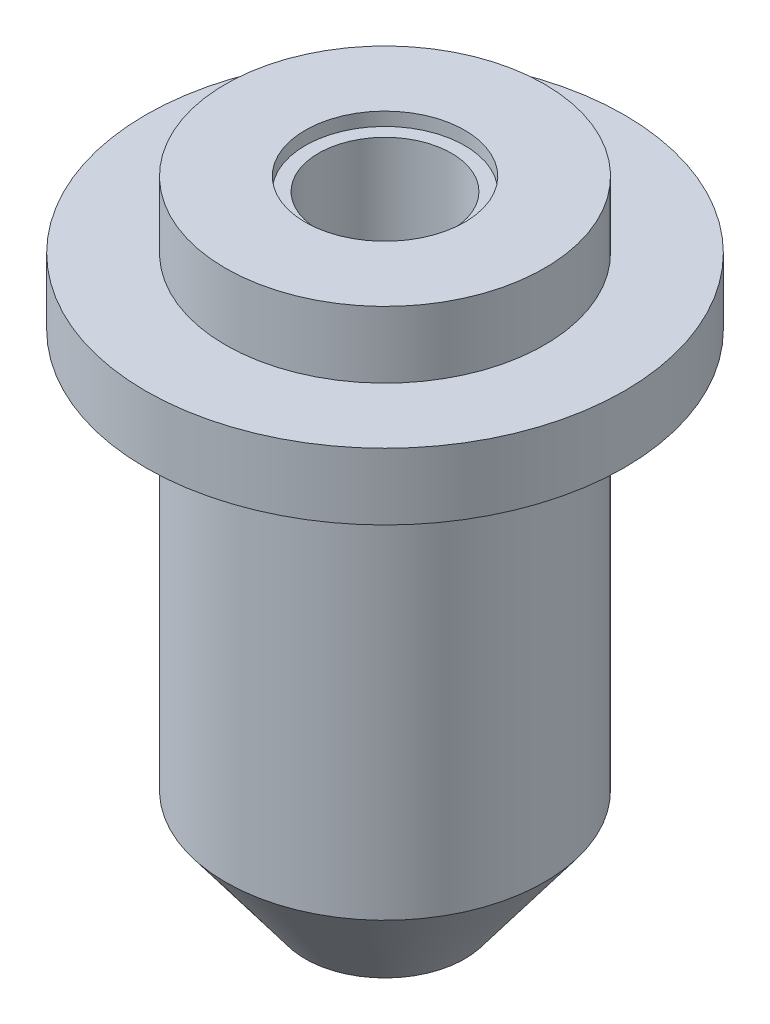
ISO-10303-21;
HEADER;
FILE_DESCRIPTION(('STEP AP214'),'2;1');
FILE_NAME('part.step','',(''),(''),'','','');
FILE_SCHEMA(('AUTOMOTIVE_DESIGN { 1 0 10303 214 1 1 1 1 }'));
ENDSEC;
DATA;
#1=APPLICATION_CONTEXT('core data for automotive mechanical design processes');
#2=APPLICATION_PROTOCOL_DEFINITION('international standard','automotive_design',2000,#1);
#3=PRODUCT_CONTEXT('',#1,'mechanical');
#4=PRODUCT('Part','Part','',(#3));
#5=PRODUCT_RELATED_PRODUCT_CATEGORY('part','',(#4));
#6=PRODUCT_DEFINITION_FORMATION('','',#4);
#7=PRODUCT_DEFINITION_CONTEXT('part definition',#1,'design');
#8=PRODUCT_DEFINITION('design','',#6,#7);
#9=PRODUCT_DEFINITION_SHAPE('','',#8);
#10=(LENGTH_UNIT() NAMED_UNIT(*) SI_UNIT(.MILLI.,.METRE.));
#11=(NAMED_UNIT(*) PLANE_ANGLE_UNIT() SI_UNIT($,.RADIAN.));
#12=(NAMED_UNIT(*) SI_UNIT($,.STERADIAN.) SOLID_ANGLE_UNIT());
#13=UNCERTAINTY_MEASURE_WITH_UNIT(LENGTH_MEASURE(1.E-05),#10,'distance_accuracy_value','');
#14=(GEOMETRIC_REPRESENTATION_CONTEXT(3) GLOBAL_UNCERTAINTY_ASSIGNED_CONTEXT((#13)) GLOBAL_UNIT_ASSIGNED_CONTEXT((#10,
#11,#12)) REPRESENTATION_CONTEXT('',''));
#15=CARTESIAN_POINT('',(0.,0.,0.));
#16=DIRECTION('',(0.,0.,1.));
#17=DIRECTION('',(1.,0.,0.));
#18=AXIS2_PLACEMENT_3D('',#15,#16,#17);
#19=CARTESIAN_POINT('',(0.,0.,0.));
#20=DIRECTION('',(0.,1.,0.));
#21=DIRECTION('',(0.,0.,1.));
#22=AXIS2_PLACEMENT_3D('',#19,#20,#21);
#23=PLANE('',#22);
#24=CARTESIAN_POINT('',(0.,0.,0.));
#25=DIRECTION('',(0.,1.,0.));
#26=DIRECTION('',(0.,0.,1.));
#27=AXIS2_PLACEMENT_3D('',#24,#25,#26);
#28=CIRCLE('',#27,5.);
#29=CARTESIAN_POINT('',(0.,0.,5.));
#30=VERTEX_POINT('',#29);
#31=EDGE_CURVE('E73',#30,#30,#28,.T.);
#32=ORIENTED_EDGE('',*,*,#31,.T.);
#33=EDGE_LOOP('',(#32));
#34=FACE_BOUND('',#33,.T.);
#35=CARTESIAN_POINT('',(0.,0.,0.));
#36=DIRECTION('',(0.,-1.,0.));
#37=DIRECTION('',(0.,0.,-1.));
#38=AXIS2_PLACEMENT_3D('',#35,#36,#37);
#39=CIRCLE('',#38,6.);
#40=CARTESIAN_POINT('',(0.,0.,-6.));
#41=VERTEX_POINT('',#40);
#42=EDGE_CURVE('E10',#41,#41,#39,.T.);
#43=ORIENTED_EDGE('',*,*,#42,.T.);
#44=EDGE_LOOP('',(#43));
#45=FACE_BOUND('',#44,.T.);
#46=ADVANCED_FACE('F43',(#34,#45),#23,.F.);
#47=CARTESIAN_POINT('',(0.,8.,0.));
#48=DIRECTION('',(0.,1.,0.));
#49=DIRECTION('',(0.,0.,1.));
#50=AXIS2_PLACEMENT_3D('',#47,#48,#49);
#51=CONICAL_SURFACE('',#50,12.,0.643501108793284);
#52=ORIENTED_EDGE('',*,*,#42,.F.);
#53=EDGE_LOOP('',(#52));
#54=FACE_BOUND('',#53,.T.);
#55=CARTESIAN_POINT('',(0.,8.,0.));
#56=DIRECTION('',(0.,-1.,0.));
#57=DIRECTION('',(0.,0.,-1.));
#58=AXIS2_PLACEMENT_3D('',#55,#56,#57);
#59=CIRCLE('',#58,12.);
#60=CARTESIAN_POINT('',(0.,8.,-12.));
#61=VERTEX_POINT('',#60);
#62=EDGE_CURVE('E47',#61,#61,#59,.T.);
#63=ORIENTED_EDGE('',*,*,#62,.T.);
#64=EDGE_LOOP('',(#63));
#65=FACE_BOUND('',#64,.T.);
#66=ADVANCED_FACE('F125',(#54,#65),#51,.T.);
#67=CARTESIAN_POINT('',(0.,0.,0.));
#68=DIRECTION('',(0.,-1.,0.));
#69=DIRECTION('',(0.,0.,-1.));
#70=AXIS2_PLACEMENT_3D('',#67,#68,#69);
#71=CYLINDRICAL_SURFACE('',#70,12.);
#72=ORIENTED_EDGE('',*,*,#62,.F.);
#73=EDGE_LOOP('',(#72));
#74=FACE_BOUND('',#73,.T.);
#75=CARTESIAN_POINT('',(0.,38.,0.));
#76=DIRECTION('',(0.,-1.,0.));
#77=DIRECTION('',(0.,0.,-1.));
#78=AXIS2_PLACEMENT_3D('',#75,#76,#77);
#79=CIRCLE('',#78,12.);
#80=CARTESIAN_POINT('',(0.,38.,-12.));
#81=VERTEX_POINT('',#80);
#82=EDGE_CURVE('E52',#81,#81,#79,.T.);
#83=ORIENTED_EDGE('',*,*,#82,.T.);
#84=EDGE_LOOP('',(#83));
#85=FACE_BOUND('',#84,.T.);
#86=ADVANCED_FACE('F130',(#74,#85),#71,.T.);
#87=CARTESIAN_POINT('',(-12.,38.,0.));
#88=DIRECTION('',(0.,1.,0.));
#89=DIRECTION('',(0.,0.,1.));
#90=AXIS2_PLACEMENT_3D('',#87,#88,#89);
#91=PLANE('',#90);
#92=ORIENTED_EDGE('',*,*,#82,.F.);
#93=EDGE_LOOP('',(#92));
#94=FACE_BOUND('',#93,.T.);
#95=CARTESIAN_POINT('',(0.,38.,0.));
#96=DIRECTION('',(0.,-1.,0.));
#97=DIRECTION('',(0.,0.,-1.));
#98=AXIS2_PLACEMENT_3D('',#95,#96,#97);
#99=CIRCLE('',#98,18.);
#100=CARTESIAN_POINT('',(0.,38.,-18.));
#101=VERTEX_POINT('',#100);
#102=EDGE_CURVE('E60',#101,#101,#99,.T.);
#103=ORIENTED_EDGE('',*,*,#102,.T.);
#104=EDGE_LOOP('',(#103));
#105=FACE_BOUND('',#104,.T.);
#106=ADVANCED_FACE('F131',(#94,#105),#91,.F.);
#107=CARTESIAN_POINT('',(0.,0.,0.));
#108=DIRECTION('',(0.,-1.,0.));
#109=DIRECTION('',(0.,0.,-1.));
#110=AXIS2_PLACEMENT_3D('',#107,#108,#109);
#111=CYLINDRICAL_SURFACE('',#110,18.);
#112=ORIENTED_EDGE('',*,*,#102,.F.);
#113=EDGE_LOOP('',(#112));
#114=FACE_BOUND('',#113,.T.);
#115=CARTESIAN_POINT('',(0.,43.,0.));
#116=DIRECTION('',(0.,-1.,0.));
#117=DIRECTION('',(0.,0.,-1.));
#118=AXIS2_PLACEMENT_3D('',#115,#116,#117);
#119=CIRCLE('',#118,18.);
#120=CARTESIAN_POINT('',(0.,43.,-18.));
#121=VERTEX_POINT('',#120);
#122=EDGE_CURVE('E61',#121,#121,#119,.T.);
#123=ORIENTED_EDGE('',*,*,#122,.T.);
#124=EDGE_LOOP('',(#123));
#125=FACE_BOUND('',#124,.T.);
#126=ADVANCED_FACE('F116',(#114,#125),#111,.T.);
#127=CARTESIAN_POINT('',(-18.,43.,0.));
#128=DIRECTION('',(0.,-1.,0.));
#129=DIRECTION('',(0.,0.,-1.));
#130=AXIS2_PLACEMENT_3D('',#127,#128,#129);
#131=PLANE('',#130);
#132=ORIENTED_EDGE('',*,*,#122,.F.);
#133=EDGE_LOOP('',(#132));
#134=FACE_BOUND('',#133,.T.);
#135=CARTESIAN_POINT('',(0.,43.,0.));
#136=DIRECTION('',(0.,-1.,0.));
#137=DIRECTION('',(0.,0.,-1.));
#138=AXIS2_PLACEMENT_3D('',#135,#136,#137);
#139=CIRCLE('',#138,12.);
#140=CARTESIAN_POINT('',(0.,43.,-12.));
#141=VERTEX_POINT('',#140);
#142=EDGE_CURVE('E62',#141,#141,#139,.T.);
#143=ORIENTED_EDGE('',*,*,#142,.T.);
#144=EDGE_LOOP('',(#143));
#145=FACE_BOUND('',#144,.T.);
#146=ADVANCED_FACE('F112',(#134,#145),#131,.F.);
#147=CARTESIAN_POINT('',(0.,0.,0.));
#148=DIRECTION('',(0.,-1.,0.));
#149=DIRECTION('',(0.,0.,-1.));
#150=AXIS2_PLACEMENT_3D('',#147,#148,#149);
#151=CYLINDRICAL_SURFACE('',#150,12.);
#152=ORIENTED_EDGE('',*,*,#142,.F.);
#153=EDGE_LOOP('',(#152));
#154=FACE_BOUND('',#153,.T.);
#155=CARTESIAN_POINT('',(0.,48.,0.));
#156=DIRECTION('',(0.,-1.,0.));
#157=DIRECTION('',(0.,0.,-1.));
#158=AXIS2_PLACEMENT_3D('',#155,#156,#157);
#159=CIRCLE('',#158,12.);
#160=CARTESIAN_POINT('',(0.,48.,-12.));
#161=VERTEX_POINT('',#160);
#162=EDGE_CURVE('E66',#161,#161,#159,.T.);
#163=ORIENTED_EDGE('',*,*,#162,.T.);
#164=EDGE_LOOP('',(#163));
#165=FACE_BOUND('',#164,.T.);
#166=ADVANCED_FACE('F106',(#154,#165),#151,.T.);
#167=CARTESIAN_POINT('',(-12.,48.,0.));
#168=DIRECTION('',(0.,-1.,0.));
#169=DIRECTION('',(0.,0.,-1.));
#170=AXIS2_PLACEMENT_3D('',#167,#168,#169);
#171=PLANE('',#170);
#172=CARTESIAN_POINT('',(0.,48.,0.));
#173=DIRECTION('',(0.,1.,0.));
#174=DIRECTION('',(0.,0.,1.));
#175=AXIS2_PLACEMENT_3D('',#172,#173,#174);
#176=CIRCLE('',#175,6.);
#177=CARTESIAN_POINT('',(0.,48.,6.));
#178=VERTEX_POINT('',#177);
#179=EDGE_CURVE('E75',#178,#178,#176,.T.);
#180=ORIENTED_EDGE('',*,*,#179,.F.);
#181=EDGE_LOOP('',(#180));
#182=FACE_BOUND('',#181,.T.);
#183=ORIENTED_EDGE('',*,*,#162,.F.);
#184=EDGE_LOOP('',(#183));
#185=FACE_BOUND('',#184,.T.);
#186=ADVANCED_FACE('F99',(#182,#185),#171,.F.);
#187=CARTESIAN_POINT('',(0.,47.,0.));
#188=DIRECTION('',(0.,1.,0.));
#189=DIRECTION('',(0.,0.,1.));
#190=AXIS2_PLACEMENT_3D('',#187,#188,#189);
#191=CYLINDRICAL_SURFACE('',#190,6.);
#192=CARTESIAN_POINT('',(0.,47.,0.));
#193=DIRECTION('',(0.,1.,0.));
#194=DIRECTION('',(0.,0.,1.));
#195=AXIS2_PLACEMENT_3D('',#192,#193,#194);
#196=CIRCLE('',#195,6.);
#197=CARTESIAN_POINT('',(0.,47.,6.));
#198=VERTEX_POINT('',#197);
#199=EDGE_CURVE('E72',#198,#198,#196,.T.);
#200=ORIENTED_EDGE('',*,*,#199,.F.);
#201=EDGE_LOOP('',(#200));
#202=FACE_BOUND('',#201,.T.);
#203=ORIENTED_EDGE('',*,*,#179,.T.);
#204=EDGE_LOOP('',(#203));
#205=FACE_BOUND('',#204,.T.);
#206=ADVANCED_FACE('F94',(#202,#205),#191,.F.);
#207=CARTESIAN_POINT('',(0.,47.,0.));
#208=DIRECTION('',(0.,1.,0.));
#209=DIRECTION('',(0.,0.,1.));
#210=AXIS2_PLACEMENT_3D('',#207,#208,#209);
#211=PLANE('',#210);
#212=CARTESIAN_POINT('',(0.,47.,0.));
#213=DIRECTION('',(0.,1.,0.));
#214=DIRECTION('',(0.,0.,1.));
#215=AXIS2_PLACEMENT_3D('',#212,#213,#214);
#216=CIRCLE('',#215,5.);
#217=CARTESIAN_POINT('',(0.,47.,5.));
#218=VERTEX_POINT('',#217);
#219=EDGE_CURVE('E80',#218,#218,#216,.T.);
#220=ORIENTED_EDGE('',*,*,#219,.F.);
#221=EDGE_LOOP('',(#220));
#222=FACE_BOUND('',#221,.T.);
#223=ORIENTED_EDGE('',*,*,#199,.T.);
#224=EDGE_LOOP('',(#223));
#225=FACE_BOUND('',#224,.T.);
#226=ADVANCED_FACE('F86',(#222,#225),#211,.T.);
#227=CARTESIAN_POINT('',(0.,0.,0.));
#228=DIRECTION('',(0.,1.,0.));
#229=DIRECTION('',(0.,0.,1.));
#230=AXIS2_PLACEMENT_3D('',#227,#228,#229);
#231=CYLINDRICAL_SURFACE('',#230,5.);
#232=ORIENTED_EDGE('',*,*,#31,.F.);
#233=EDGE_LOOP('',(#232));
#234=FACE_BOUND('',#233,.T.);
#235=ORIENTED_EDGE('',*,*,#219,.T.);
#236=EDGE_LOOP('',(#235));
#237=FACE_BOUND('',#236,.T.);
#238=ADVANCED_FACE('F84',(#234,#237),#231,.F.);
#239=CLOSED_SHELL('',(#46,#66,#86,#106,#126,#146,#166,#186,#206,#226,#238));
#240=MANIFOLD_SOLID_BREP('B2',#239);
#241=ADVANCED_BREP_SHAPE_REPRESENTATION('',(#18,#240),#14);
#242=SHAPE_DEFINITION_REPRESENTATION(#9,#241);
ENDSEC;
END-ISO-10303-21;
